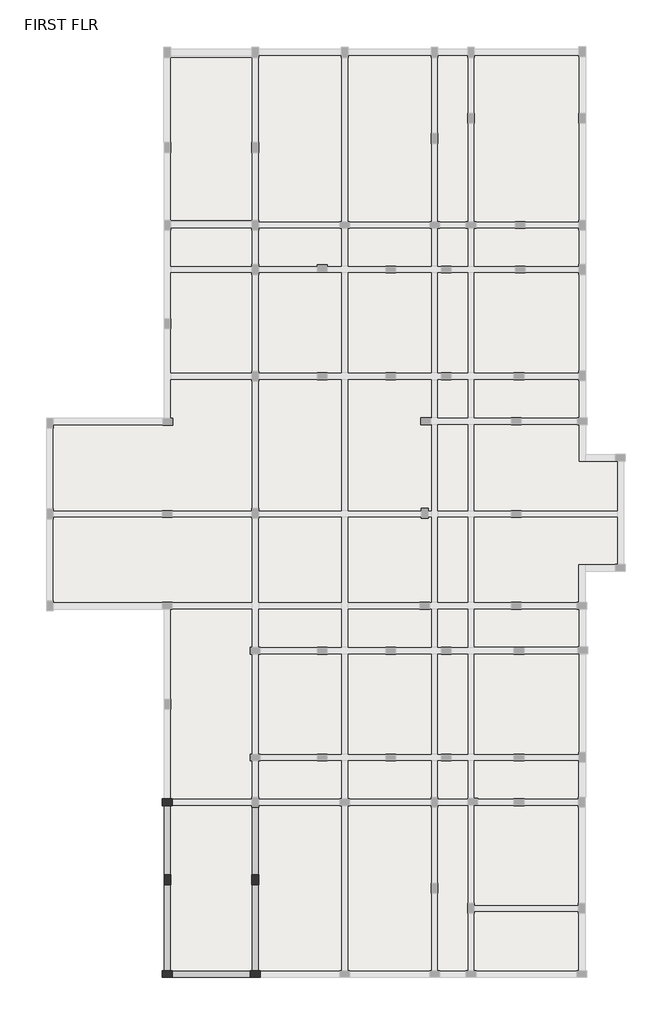
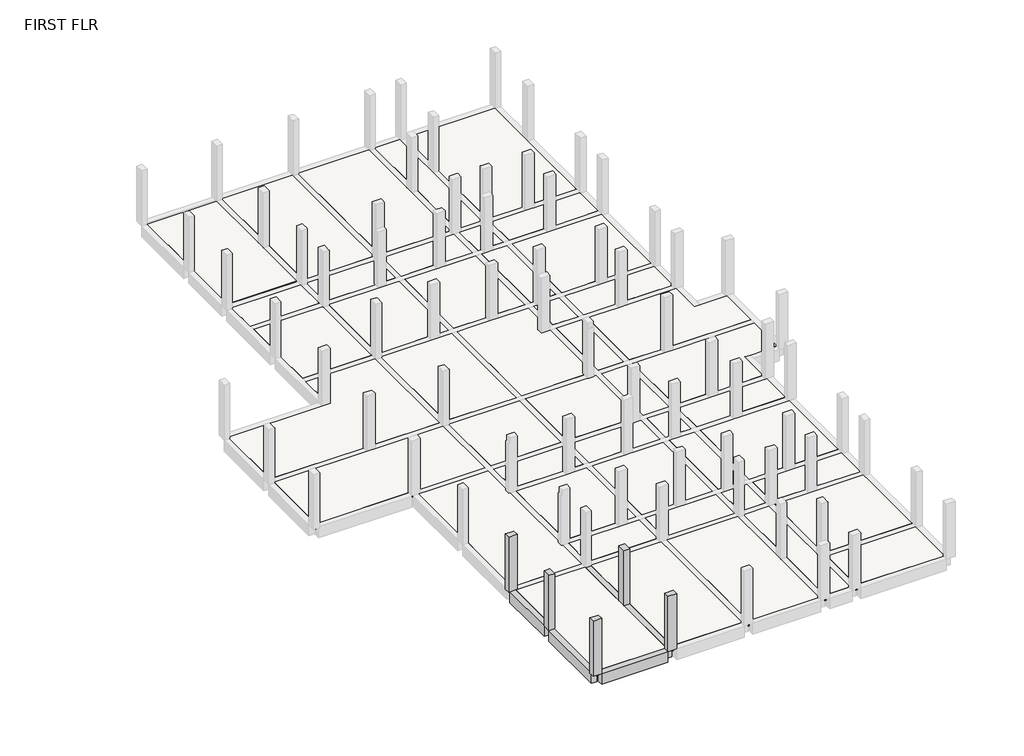
# One storey, part 1 of 5: 5 beams, 5 columns, 2 slabs.
"""IFC4 building model written with IfcOpenShell, lengths in millimetres."""

from ifc_helpers import new_model, si_unit, frame, origin, place, context, project, spatial, polyline, outline, extrude, faceted_brep, element, save

model = new_model("IFC4")

# Units and contexts
model_context = context("Model", 3, world=origin())
ifc_project = project(units=[si_unit("LENGTHUNIT", "METRE", prefix="MILLI")], contexts=[model_context])

# Site, building, storey
site = spatial("IfcSite", under=ifc_project)
building = spatial("IfcBuilding", under=site)
storey = spatial("IfcBuildingStorey", under=building, Name="FIRST FLR", Elevation=3000.0)

# Beams
placement = place(None, origin())
element("IfcBeam", 1, ObjectType="M_Concrete-Rectangular Beam : 300 x 600mm", at=placement, inside=storey, context=model_context, shape_type="Brep", body=[
    faceted_brep([(-5588.8105653, -14991.2517597, 3000.0), (-5588.8105653, -11907.8970059, 3000.0), (-5888.8105653, -11907.8970059, 3000.0), (-5888.8105653, -14991.2517597, 3000.0), (-5888.8105653, -11907.8970059, 2400.0), (-5888.8105653, -14991.2517597, 2400.0), (-5588.8105653, -11907.8970059, 2400.0), (-5588.8105653, -14991.2517597, 2400.0), (-5588.8105653, -14991.2517597, 2700.0), (-5588.8105653, -11907.8970059, 2700.0)], [[[0, 1, 2, 3]], [[3, 2, 4, 5]], [[5, 4, 6, 7]], [[1, 0, 8, 7, 6, 9]], [[6, 4, 2, 1, 9]], [[0, 3, 5, 7, 8]]]),
])
element("IfcBeam", 2, ObjectType="M_Concrete-Rectangular Beam : 300 x 600mm", at=placement, inside=storey, context=model_context, shape_type="Brep", body=[
    faceted_brep([(-5588.8105653, -15441.2517597, 3000.0), (-5888.8105653, -15441.2517597, 3000.0), (-5888.8105653, -19272.5304373, 3000.0), (-5588.8105653, -19272.5304373, 3000.0), (-5888.8105653, -15441.2517597, 2400.0), (-5888.8105653, -19272.5304373, 2400.0), (-5588.8105653, -15441.2517597, 2400.0), (-5588.8105653, -19272.5304373, 2400.0), (-5588.8105653, -19272.5304373, 2700.0), (-5588.8105653, -15441.2517597, 2700.0)], [[[0, 1, 2, 3]], [[1, 4, 5, 2]], [[4, 6, 7, 5]], [[0, 3, 8, 7, 6, 9]], [[6, 4, 1, 0, 9]], [[3, 2, 5, 7, 8]]]),
])
element("IfcBeam", 3, ObjectType="M_Concrete-Rectangular Beam : 300 x 600mm", at=placement, inside=storey, context=model_context, shape_type="SweptSolid", body=[
    extrude(outline(polyline([(-2046.7865686, -19272.5304373), (-2046.7865686, -19572.5304373), (-5516.7865686, -19572.5304373), (-5516.7865686, -19272.5304373), (-2046.7865686, -19272.5304373)])), frame((0.0, 0.0, 2400.0), z_axis=(0.0, 0.0, 1.0), x_axis=(1.0, 0.0, 0.0)), (0.0, 0.0, 1.0), 600.0),
])
element("IfcBeam", 4, ObjectType="M_Concrete-Rectangular Beam : 300 x 600mm", at=placement, inside=storey, context=model_context, shape_type="Brep", body=[
    faceted_brep([(-1971.7865686, -15441.2517597, 3000.0), (-1971.7865686, -19272.5304373, 3000.0), (-1671.7865686, -19272.5304373, 3000.0), (-1671.7865686, -15441.2517597, 3000.0), (-1671.7865686, -19272.5304373, 2700.0), (-1671.7865686, -19272.5304373, 2400.0), (-1671.7865686, -15441.2517597, 2400.0), (-1671.7865686, -15441.2517597, 2700.0), (-1971.7865686, -19272.5304373, 2400.0), (-1971.7865686, -15441.2517597, 2400.0), (-1971.7865686, -15441.2517597, 2700.0), (-1971.7865686, -19272.5304373, 2700.0)], [[[0, 1, 2, 3]], [[3, 2, 4, 5, 6, 7]], [[6, 5, 8, 9]], [[1, 0, 10, 9, 8, 11]], [[0, 3, 7, 6, 9, 10]], [[8, 5, 4, 2, 1, 11]]]),
])
element("IfcBeam", 5, ObjectType="M_Concrete-Rectangular Beam : 300 x 600mm", at=placement, inside=storey, context=model_context, shape_type="Brep", body=[
    faceted_brep([(-1971.7865686, -11982.8970059, 3000.0), (-1971.7865686, -14991.2517597, 3000.0), (-1671.7865686, -14991.2517597, 3000.0), (-1671.7865686, -11982.8970059, 3000.0), (-1671.7865686, -14991.2517597, 2700.0), (-1671.7865686, -14991.2517597, 2400.0), (-1671.7865686, -11982.8970059, 2400.0), (-1671.7865686, -11982.8970059, 2700.0), (-1971.7865686, -14991.2517597, 2400.0), (-1971.7865686, -11982.8970059, 2400.0), (-1971.7865686, -11982.8970059, 2700.0), (-1971.7865686, -14991.2517597, 2700.0)], [[[0, 1, 2, 3]], [[3, 2, 4, 5, 6, 7]], [[6, 5, 8, 9]], [[1, 0, 10, 9, 8, 11]], [[0, 3, 7, 6, 9, 10]], [[8, 5, 4, 2, 1, 11]]]),
])

# Columns
element("IfcColumn", 6, ObjectType="M_Concrete-Rectangular-Column : 300 x 450mm", at=placement, inside=storey, context=model_context, shape_type="Brep", body=[
    faceted_brep([(-5513.8105653, -11907.8970059, 3000.0), (-5963.8105653, -11907.8970059, 3000.0), (-5963.8105653, -11607.8970059, 3000.0), (-5513.8105653, -11607.8970059, 3000.0), (-5513.8105653, -11907.8970059, 5748.0), (-5513.8105653, -11907.8970059, 6048.0), (-5588.8105653, -11907.8970059, 6048.0), (-5963.8105653, -11907.8970059, 6048.0), (-5963.8105653, -11607.8970059, 6048.0), (-5588.8105653, -11607.8970059, 6048.0), (-5513.8105653, -11607.8970059, 6048.0), (-5513.8105653, -11607.8970059, 5748.0)], [[[0, 1, 2, 3]], [[1, 0, 4, 5, 6, 7]], [[2, 1, 7, 8]], [[3, 2, 8, 9, 10, 11]], [[0, 3, 11, 10, 5, 4]], [[8, 7, 6, 5, 10, 9]]]),
])
element("IfcColumn", 7, ObjectType="M_Concrete-Rectangular-Column : 300 x 450mm", at=placement, inside=storey, context=model_context, shape_type="Brep", body=[
    faceted_brep([(-5588.8105653, -14991.2517597, 3000.0), (-5588.8105653, -15441.2517597, 3000.0), (-5888.8105653, -15441.2517597, 3000.0), (-5888.8105653, -14991.2517597, 3000.0), (-5588.8105653, -14991.2517597, 5748.0), (-5588.8105653, -14991.2517597, 6048.0), (-5588.8105653, -15441.2517597, 6048.0), (-5588.8105653, -15441.2517597, 5748.0), (-5888.8105653, -15441.2517597, 6048.0), (-5888.8105653, -14991.2517597, 6048.0)], [[[0, 1, 2, 3]], [[1, 0, 4, 5, 6, 7]], [[2, 1, 7, 6, 8]], [[3, 2, 8, 9]], [[0, 3, 9, 5, 4]], [[6, 5, 9, 8]]]),
])
element("IfcColumn", 8, ObjectType="M_Concrete-Rectangular-Column : 300 x 450mm", at=placement, inside=storey, context=model_context, shape_type="Brep", body=[
    faceted_brep([(-1671.7865686, -14991.2517597, 3000.0), (-1671.7865686, -15441.2517597, 3000.0), (-1971.7865686, -15441.2517597, 3000.0), (-1971.7865686, -14991.2517597, 3000.0), (-1671.7865686, -14991.2517597, 5748.0), (-1671.7865686, -14991.2517597, 6048.0), (-1671.7865686, -15441.2517597, 6048.0), (-1671.7865686, -15441.2517597, 5748.0), (-1971.7865686, -15441.2517597, 6048.0), (-1971.7865686, -15441.2517597, 5748.0), (-1971.7865686, -14991.2517597, 6048.0), (-1971.7865686, -14991.2517597, 5748.0)], [[[0, 1, 2, 3]], [[1, 0, 4, 5, 6, 7]], [[2, 1, 7, 6, 8, 9]], [[3, 2, 9, 8, 10, 11]], [[0, 3, 11, 10, 5, 4]], [[6, 5, 10, 8]]]),
])
element("IfcColumn", 9, ObjectType="M_Concrete-Rectangular-Column : 300 x 450mm", at=placement, inside=storey, context=model_context, shape_type="Brep", body=[
    faceted_brep([(-2046.7865686, -19272.5304373, 3000.0), (-1596.7865686, -19272.5304373, 3000.0), (-1596.7865686, -19572.5304373, 3000.0), (-2046.7865686, -19572.5304373, 3000.0), (-2046.7865686, -19272.5304373, 6048.0), (-1971.7865686, -19272.5304373, 6048.0), (-1671.7865686, -19272.5304373, 6048.0), (-1596.7865686, -19272.5304373, 6048.0), (-1596.7865686, -19572.5304373, 6048.0), (-2046.7865686, -19572.5304373, 6048.0)], [[[0, 1, 2, 3]], [[4, 5, 6, 7, 1, 0]], [[7, 8, 2, 1]], [[8, 9, 3, 2]], [[9, 4, 0, 3]], [[4, 9, 8, 7, 6, 5]]]),
])
element("IfcColumn", 10, ObjectType="M_Concrete-Rectangular-Column : 300 x 450mm", at=placement, inside=storey, context=model_context, shape_type="Brep", body=[
    faceted_brep([(-5516.7865686, -19572.5304373, 3000.0), (-5966.7865686, -19572.5304373, 3000.0), (-5966.7865686, -19272.5304373, 3000.0), (-5516.7865686, -19272.5304373, 3000.0), (-5516.7865686, -19572.5304373, 6048.0), (-5966.7865686, -19572.5304373, 6048.0), (-5966.7865686, -19272.5304373, 6048.0), (-5588.8105653, -19272.5304373, 6048.0), (-5516.7865686, -19272.5304373, 6048.0)], [[[0, 1, 2, 3]], [[4, 5, 1, 0]], [[5, 6, 2, 1]], [[6, 7, 8, 3, 2]], [[8, 4, 0, 3]], [[4, 8, 7, 6, 5]]]),
])

# Slabs
element("IfcSlab", 11, ObjectType="Generic 300mm", at=placement, inside=storey, context=model_context, shape_type="Brep", body=[
    faceted_brep([(-1971.7865686, 21462.8349362, 2700.0), (-1971.7865686, 14212.5179708, 2700.0), (-5588.8105653, 14212.5179708, 2700.0), (-5591.7865686, 14212.5179708, 2700.0), (-5591.7865686, 17224.7148651, 2700.0), (-5591.7865686, 17674.7148651, 2700.0), (-5591.7865686, 21462.8349362, 2700.0), (-1971.7865686, 21462.8349362, 3000.0), (-5591.7865686, 21462.8349362, 3000.0), (-5591.7865686, 17674.7148651, 3000.0), (-5591.7865686, 17224.7148651, 3000.0), (-5591.7865686, 14212.5179708, 3000.0), (-5588.8105653, 14212.5179708, 3000.0), (-1971.7865686, 14212.5179708, 3000.0), (-1971.7865686, 17224.7148651, 3000.0), (-1971.7865686, 17674.7148651, 3000.0)], [[[0, 1, 2, 3, 4, 5, 6]], [[7, 8, 9, 10, 11, 12, 13, 14, 15]], [[1, 0, 7, 15, 14, 13]], [[3, 2, 1, 13, 12, 11]], [[6, 5, 4, 3, 11, 10, 9, 8]], [[0, 6, 8, 7]]]),
    faceted_brep([(2024.7296816, 21537.8349362, 2700.0), (2024.7296816, 14137.5179708, 2700.0), (-1671.7865686, 14137.5179708, 2700.0), (-1671.7865686, 21537.8349362, 2700.0), (2024.7296816, 21537.8349362, 3000.0), (-1671.7865686, 21537.8349362, 3000.0), (-1671.7865686, 21462.8349362, 3000.0), (-1671.7865686, 17674.7148651, 3000.0), (-1671.7865686, 17224.7148651, 3000.0), (-1671.7865686, 14212.5179708, 3000.0), (-1671.7865686, 14137.5179708, 3000.0), (1949.7296816, 14137.5179708, 3000.0), (2024.7296816, 14137.5179708, 3000.0), (2024.7296816, 21462.8349362, 3000.0)], [[[0, 1, 2, 3]], [[4, 5, 6, 7, 8, 9, 10, 11, 12, 13]], [[1, 0, 4, 13, 12]], [[2, 1, 12, 11, 10]], [[3, 2, 10, 9, 8, 7, 6, 5]], [[0, 3, 5, 4]]]),
    faceted_brep([(6032.5248054, 21537.8349362, 2700.0), (6032.5248054, 14137.5179708, 2700.0), (2324.7296816, 14137.5179708, 2700.0), (2324.7296816, 21537.8349362, 2700.0), (6032.5248054, 21537.8349362, 3000.0), (2324.7296816, 21537.8349362, 3000.0), (2324.7296816, 21462.8349362, 3000.0), (2324.7296816, 14137.5179708, 3000.0), (2399.7296816, 14137.5179708, 3000.0), (5957.5248054, 14137.5179708, 3000.0), (6032.5248054, 14137.5179708, 3000.0), (6032.5248054, 17624.7148651, 3000.0), (6032.5248054, 18074.7148651, 3000.0), (6032.5248054, 21462.8349362, 3000.0)], [[[0, 1, 2, 3]], [[4, 5, 6, 7, 8, 9, 10, 11, 12, 13]], [[1, 0, 4, 13, 12, 11, 10]], [[2, 1, 10, 9, 8, 7]], [[3, 2, 7, 6, 5]], [[0, 3, 5, 4]]]),
    faceted_brep([(7656.8679014, 21537.8349362, 2700.0), (7656.8679014, 14137.5179708, 2700.0), (6332.5248054, 14137.5179708, 2700.0), (6332.5248054, 21537.8349362, 2700.0), (7656.8679014, 21537.8349362, 3000.0), (6332.5248054, 21537.8349362, 3000.0), (6332.5248054, 21462.8349362, 3000.0), (6332.5248054, 18074.7148651, 3000.0), (6332.5248054, 17624.7148651, 3000.0), (6332.5248054, 14137.5179708, 3000.0), (6407.5248054, 14137.5179708, 3000.0), (7581.8679014, 14137.5179708, 3000.0), (7656.8679014, 14137.5179708, 3000.0), (7656.8679014, 18524.7148651, 3000.0), (7656.8679014, 18974.7148651, 3000.0), (7656.8679014, 21462.8349362, 3000.0)], [[[0, 1, 2, 3]], [[4, 5, 6, 7, 8, 9, 10, 11, 12, 13, 14, 15]], [[1, 0, 4, 15, 14, 13, 12]], [[2, 1, 12, 11, 10, 9]], [[3, 2, 9, 8, 7, 6, 5]], [[0, 3, 5, 4]]]),
    faceted_brep([(12619.1163908, 21537.8349362, 2700.0), (12619.1163908, 14137.5179708, 2700.0), (7956.8679014, 14137.5179708, 2700.0), (7956.8679014, 21537.8349362, 2700.0), (12619.1163908, 21537.8349362, 3000.0), (7956.8679014, 21537.8349362, 3000.0), (7956.8679014, 21462.8349362, 3000.0), (7956.8679014, 18974.7148651, 3000.0), (7956.8679014, 18524.7148651, 3000.0), (7956.8679014, 14137.5179708, 3000.0), (8031.8679014, 14137.5179708, 3000.0), (9781.8679014, 14137.5179708, 3000.0), (10231.8679014, 14137.5179708, 3000.0), (12619.1163908, 14137.5179708, 3000.0), (12619.1163908, 14212.5179708, 3000.0), (12619.1163908, 18524.7148651, 3000.0), (12619.1163908, 18974.7148651, 3000.0), (12619.1163908, 21502.8349362, 3000.0)], [[[0, 1, 2, 3]], [[4, 5, 6, 7, 8, 9, 10, 11, 12, 13, 14, 15, 16, 17]], [[1, 0, 4, 17, 16, 15, 14, 13]], [[2, 1, 13, 12, 11, 10, 9]], [[3, 2, 9, 8, 7, 6, 5]], [[0, 3, 5, 4]]]),
    faceted_brep([(-1971.7865686, 13837.5179708, 2700.0), (-1971.7865686, 12157.4075451, 2700.0), (-5588.8105653, 12157.4075451, 2700.0), (-5588.8105653, 13837.5179708, 2700.0), (-1971.7865686, 13837.5179708, 3000.0), (-5588.8105653, 13837.5179708, 3000.0), (-5588.8105653, 13762.5179708, 3000.0), (-5588.8105653, 12157.4075451, 3000.0), (-1971.7865686, 12157.4075451, 3000.0), (-1971.7865686, 12232.4075451, 3000.0), (-1971.7865686, 13762.5179708, 3000.0)], [[[0, 1, 2, 3]], [[4, 5, 6, 7, 8, 9, 10]], [[1, 0, 4, 10, 9, 8]], [[2, 1, 8, 7]], [[3, 2, 7, 6, 5]], [[0, 3, 5, 4]]]),
    faceted_brep([(2024.7296816, 13837.5179708, 2700.0), (2024.7296816, 12157.4075451, 2700.0), (1399.7296816, 12157.4075451, 2700.0), (949.7296816, 12157.4075451, 2700.0), (-1671.7865686, 12157.4075451, 2700.0), (-1671.7865686, 13837.5179708, 2700.0), (2024.7296816, 13837.5179708, 3000.0), (1949.7296816, 13837.5179708, 3000.0), (-1671.7865686, 13837.5179708, 3000.0), (-1671.7865686, 13762.5179708, 3000.0), (-1671.7865686, 12232.4075451, 3000.0), (-1671.7865686, 12157.4075451, 3000.0), (949.7296816, 12157.4075451, 3000.0), (1399.7296816, 12157.4075451, 3000.0), (2024.7296816, 12157.4075451, 3000.0)], [[[0, 1, 2, 3, 4, 5]], [[6, 7, 8, 9, 10, 11, 12, 13, 14]], [[1, 0, 6, 14]], [[4, 3, 2, 1, 14, 13, 12, 11]], [[5, 4, 11, 10, 9, 8]], [[0, 5, 8, 7, 6]]]),
    faceted_brep([(6032.5248054, 13837.5179708, 2700.0), (6032.5248054, 12157.4075451, 2700.0), (2324.7296816, 12157.4075451, 2700.0), (2324.7296816, 13837.5179708, 2700.0), (6032.5248054, 13837.5179708, 3000.0), (5957.5248054, 13837.5179708, 3000.0), (2399.7296816, 13837.5179708, 3000.0), (2324.7296816, 13837.5179708, 3000.0), (2324.7296816, 12157.4075451, 3000.0), (3997.5248054, 12157.4075451, 3000.0), (4447.5248054, 12157.4075451, 3000.0), (6032.5248054, 12157.4075451, 3000.0)], [[[0, 1, 2, 3]], [[4, 5, 6, 7, 8, 9, 10, 11]], [[1, 0, 4, 11]], [[2, 1, 11, 10, 9, 8]], [[3, 2, 8, 7]], [[0, 3, 7, 6, 5, 4]]]),
    faceted_brep([(7656.8679014, 13837.5179708, 2700.0), (7656.8679014, 12157.4075451, 2700.0), (6332.5248054, 12157.4075451, 2700.0), (6332.5248054, 13837.5179708, 2700.0), (7656.8679014, 13837.5179708, 3000.0), (7581.8679014, 13837.5179708, 3000.0), (6407.5248054, 13837.5179708, 3000.0), (6332.5248054, 13837.5179708, 3000.0), (6332.5248054, 12157.4075451, 3000.0), (6481.8679014, 12157.4075451, 3000.0), (6931.8679014, 12157.4075451, 3000.0), (7656.8679014, 12157.4075451, 3000.0)], [[[0, 1, 2, 3]], [[4, 5, 6, 7, 8, 9, 10, 11]], [[1, 0, 4, 11]], [[2, 1, 11, 10, 9, 8]], [[3, 2, 8, 7]], [[0, 3, 7, 6, 5, 4]]]),
    faceted_brep([(12619.1163908, 13837.5179708, 2700.0), (12619.1163908, 12157.4075451, 2700.0), (7956.8679014, 12157.4075451, 2700.0), (7956.8679014, 13837.5179708, 2700.0), (12619.1163908, 13837.5179708, 3000.0), (10231.8679014, 13837.5179708, 3000.0), (9781.8679014, 13837.5179708, 3000.0), (8031.8679014, 13837.5179708, 3000.0), (7956.8679014, 13837.5179708, 3000.0), (7956.8679014, 12157.4075451, 3000.0), (9781.8679014, 12157.4075451, 3000.0), (10231.8679014, 12157.4075451, 3000.0), (12619.1163908, 12157.4075451, 3000.0), (12619.1163908, 12232.4075451, 3000.0), (12619.1163908, 13762.5179708, 3000.0)], [[[0, 1, 2, 3]], [[4, 5, 6, 7, 8, 9, 10, 11, 12, 13, 14]], [[1, 0, 4, 14, 13, 12]], [[2, 1, 12, 11, 10, 9]], [[3, 2, 9, 8]], [[0, 3, 8, 7, 6, 5, 4]]]),
    faceted_brep([(-1971.7865686, 11857.4075451, 2700.0), (-1971.7865686, 7399.7076276, 2700.0), (-5588.8105653, 7399.7076276, 2700.0), (-5588.8105653, 11857.4075451, 2700.0), (-1971.7865686, 11857.4075451, 3000.0), (-5588.8105653, 11857.4075451, 3000.0), (-5588.8105653, 9817.5252033, 3000.0), (-5588.8105653, 9367.5252033, 3000.0), (-5588.8105653, 7399.7076276, 3000.0), (-1971.7865686, 7399.7076276, 3000.0), (-1971.7865686, 7474.7076276, 3000.0), (-1971.7865686, 11782.4075451, 3000.0)], [[[0, 1, 2, 3]], [[4, 5, 6, 7, 8, 9, 10, 11]], [[1, 0, 4, 11, 10, 9]], [[2, 1, 9, 8]], [[3, 2, 8, 7, 6, 5]], [[0, 3, 5, 4]]]),
    faceted_brep([(2024.7296816, 11857.4075451, 2700.0), (2024.7296816, 7399.7076276, 2700.0), (-1671.7865686, 7399.7076276, 2700.0), (-1671.7865686, 11857.4075451, 2700.0), (2024.7296816, 11857.4075451, 3000.0), (-1671.7865686, 11857.4075451, 3000.0), (-1671.7865686, 11782.4075451, 3000.0), (-1671.7865686, 7474.7076276, 3000.0), (-1671.7865686, 7399.7076276, 3000.0), (949.7296816, 7399.7076276, 3000.0), (1399.7296816, 7399.7076276, 3000.0), (2024.7296816, 7399.7076276, 3000.0)], [[[0, 1, 2, 3]], [[4, 5, 6, 7, 8, 9, 10, 11]], [[1, 0, 4, 11]], [[2, 1, 11, 10, 9, 8]], [[3, 2, 8, 7, 6, 5]], [[0, 3, 5, 4]]]),
    faceted_brep([(6032.5248054, 11857.4075451, 2700.0), (6032.5248054, 7399.7076276, 2700.0), (2324.7296816, 7399.7076276, 2700.0), (2324.7296816, 11857.4075451, 2700.0), (6032.5248054, 11857.4075451, 3000.0), (4447.5248054, 11857.4075451, 3000.0), (3997.5248054, 11857.4075451, 3000.0), (2324.7296816, 11857.4075451, 3000.0), (2324.7296816, 7399.7076276, 3000.0), (3997.5248054, 7399.7076276, 3000.0), (4447.5248054, 7399.7076276, 3000.0), (6032.5248054, 7399.7076276, 3000.0)], [[[0, 1, 2, 3]], [[4, 5, 6, 7, 8, 9, 10, 11]], [[1, 0, 4, 11]], [[2, 1, 11, 10, 9, 8]], [[3, 2, 8, 7]], [[0, 3, 7, 6, 5, 4]]]),
    faceted_brep([(7656.8679014, 11857.4075451, 2700.0), (7656.8679014, 7399.7076276, 2700.0), (6332.5248054, 7399.7076276, 2700.0), (6332.5248054, 11857.4075451, 2700.0), (7656.8679014, 11857.4075451, 3000.0), (6931.8679014, 11857.4075451, 3000.0), (6481.8679014, 11857.4075451, 3000.0), (6332.5248054, 11857.4075451, 3000.0), (6332.5248054, 7399.7076276, 3000.0), (6481.8679014, 7399.7076276, 3000.0), (6931.8679014, 7399.7076276, 3000.0), (7656.8679014, 7399.7076276, 3000.0)], [[[0, 1, 2, 3]], [[4, 5, 6, 7, 8, 9, 10, 11]], [[1, 0, 4, 11]], [[2, 1, 11, 10, 9, 8]], [[3, 2, 8, 7]], [[0, 3, 7, 6, 5, 4]]]),
    faceted_brep([(12616.8679014, 11857.4075451, 2700.0), (12616.8679014, 7399.7076276, 2700.0), (7956.8679014, 7399.7076276, 2700.0), (7956.8679014, 11857.4075451, 2700.0), (12616.8679014, 11857.4075451, 3000.0), (10231.8679014, 11857.4075451, 3000.0), (9781.8679014, 11857.4075451, 3000.0), (7956.8679014, 11857.4075451, 3000.0), (7956.8679014, 7399.7076276, 3000.0), (9721.8679014, 7399.7076276, 3000.0), (10171.8679014, 7399.7076276, 3000.0), (12616.8679014, 7399.7076276, 3000.0)], [[[0, 1, 2, 3]], [[4, 5, 6, 7, 8, 9, 10, 11]], [[1, 0, 4, 11]], [[2, 1, 11, 10, 9, 8]], [[3, 2, 8, 7]], [[0, 3, 7, 6, 5, 4]]]),
    faceted_brep([(7656.8679014, 7099.7076276, 2700.0), (7656.8679014, 5387.6057249, 2700.0), (6332.5248054, 5387.6057249, 2700.0), (6332.5248054, 7099.7076276, 2700.0), (7656.8679014, 7099.7076276, 3000.0), (6931.8679014, 7099.7076276, 3000.0), (6481.8679014, 7099.7076276, 3000.0), (6332.5248054, 7099.7076276, 3000.0), (6332.5248054, 5387.6057249, 3000.0), (7656.8679014, 5387.6057249, 3000.0)], [[[0, 1, 2, 3]], [[4, 5, 6, 7, 8, 9]], [[1, 0, 4, 9]], [[2, 1, 9, 8]], [[3, 2, 8, 7]], [[0, 3, 7, 6, 5, 4]]]),
    faceted_brep([(12616.8679014, 7099.7076276, 2700.0), (12616.8679014, 5387.6057249, 2700.0), (7956.8679014, 5387.6057249, 2700.0), (7956.8679014, 7099.7076276, 2700.0), (12616.8679014, 7099.7076276, 3000.0), (10171.8679014, 7099.7076276, 3000.0), (9721.8679014, 7099.7076276, 3000.0), (7956.8679014, 7099.7076276, 3000.0), (7956.8679014, 5387.6057249, 3000.0), (9601.8679014, 5387.6057249, 3000.0), (10051.8679014, 5387.6057249, 3000.0), (12541.8679014, 5387.6057249, 3000.0), (12616.8679014, 5387.6057249, 3000.0)], [[[0, 1, 2, 3]], [[4, 5, 6, 7, 8, 9, 10, 11, 12]], [[1, 0, 4, 12]], [[2, 1, 12, 11, 10, 9, 8]], [[3, 2, 8, 7]], [[0, 3, 7, 6, 5, 4]]]),
    faceted_brep([(7656.8679014, 5087.6057249, 2700.0), (7656.8679014, 1251.1713929, 2700.0), (6332.5248054, 1251.1713929, 2700.0), (6332.5248054, 5087.6057249, 2700.0), (7656.8679014, 5087.6057249, 3000.0), (6332.5248054, 5087.6057249, 3000.0), (6332.5248054, 1251.1713929, 3000.0), (7656.8679014, 1251.1713929, 3000.0)], [[[0, 1, 2, 3]], [[4, 5, 6, 7]], [[1, 0, 4, 7]], [[2, 1, 7, 6]], [[3, 2, 6, 5]], [[0, 3, 5, 4]]]),
    faceted_brep([(14319.1163908, 1251.1713929, 2700.0), (7956.8679014, 1251.1713929, 2700.0), (7956.8679014, 5087.6057249, 2700.0), (12616.8679014, 5087.6057249, 2700.0), (12616.8679014, 3435.7536525, 2700.0), (14319.1163908, 3435.7536525, 2700.0), (14319.1163908, 1251.1713929, 3000.0), (14319.1163908, 3435.7536525, 3000.0), (12916.8679014, 3435.7536525, 3000.0), (12616.8679014, 3435.7536525, 3000.0), (12616.8679014, 5087.6057249, 3000.0), (12541.8679014, 5087.6057249, 3000.0), (10051.8679014, 5087.6057249, 3000.0), (9601.8679014, 5087.6057249, 3000.0), (7956.8679014, 5087.6057249, 3000.0), (7956.8679014, 1251.1713929, 3000.0), (9601.8679014, 1251.1713929, 3000.0), (10051.8679014, 1251.1713929, 3000.0)], [[[0, 1, 2, 3, 4, 5]], [[6, 7, 8, 9, 10, 11, 12, 13, 14, 15, 16, 17]], [[1, 0, 6, 17, 16, 15]], [[2, 1, 15, 14]], [[3, 2, 14, 13, 12, 11, 10]], [[4, 3, 10, 9]], [[5, 4, 9, 8, 7]], [[0, 5, 7, 6]]]),
    faceted_brep([(7956.8679014, -2839.4535766, 2700.0), (7956.8679014, 951.1713929, 2700.0), (14319.1163908, 951.1713929, 2700.0), (14319.1163908, -1148.8286071, 2700.0), (12599.1163908, -1148.8286071, 2700.0), (12599.1163908, -2839.4535766, 2700.0), (7956.8679014, -2839.4535766, 3000.0), (9601.8679014, -2839.4535766, 3000.0), (10051.8679014, -2839.4535766, 3000.0), (12524.1163908, -2839.4535766, 3000.0), (12599.1163908, -2839.4535766, 3000.0), (12599.1163908, -1148.8286071, 3000.0), (12899.1163908, -1148.8286071, 3000.0), (14244.1163908, -1148.8286071, 3000.0), (14319.1163908, -1148.8286071, 3000.0), (14319.1163908, 951.1713929, 3000.0), (10051.8679014, 951.1713929, 3000.0), (9601.8679014, 951.1713929, 3000.0), (7956.8679014, 951.1713929, 3000.0)], [[[0, 1, 2, 3, 4, 5]], [[6, 7, 8, 9, 10, 11, 12, 13, 14, 15, 16, 17, 18]], [[1, 0, 6, 18]], [[2, 1, 18, 17, 16, 15]], [[3, 2, 15, 14]], [[4, 3, 14, 13, 12, 11]], [[5, 4, 11, 10]], [[0, 5, 10, 9, 8, 7, 6]]]),
    faceted_brep([(7656.8679014, 951.1713929, 2700.0), (7656.8679014, -2839.4535766, 2700.0), (6332.5248054, -2839.4535766, 2700.0), (6332.5248054, 951.1713929, 2700.0), (7656.8679014, 951.1713929, 3000.0), (6332.5248054, 951.1713929, 3000.0), (6332.5248054, -2839.4535766, 3000.0), (7656.8679014, -2839.4535766, 3000.0)], [[[0, 1, 2, 3]], [[4, 5, 6, 7]], [[1, 0, 4, 7]], [[2, 1, 7, 6]], [[3, 2, 6, 5]], [[0, 3, 5, 4]]]),
    faceted_brep([(6032.5248054, 951.1713929, 2700.0), (6032.5248054, -2839.4535766, 2700.0), (2324.7296816, -2839.4535766, 2700.0), (2324.7296816, 951.1713929, 2700.0), (5592.5248054, 951.1713929, 2700.0), (5892.5248054, 951.1713929, 2700.0), (6032.5248054, 951.1713929, 3000.0), (5892.5248054, 951.1713929, 3000.0), (5592.5248054, 951.1713929, 3000.0), (2324.7296816, 951.1713929, 3000.0), (2324.7296816, -2839.4535766, 3000.0), (5517.5248054, -2839.4535766, 3000.0), (5967.5248054, -2839.4535766, 3000.0), (6032.5248054, -2839.4535766, 3000.0)], [[[0, 1, 2, 3, 4, 5]], [[6, 7, 8, 9, 10, 11, 12, 13]], [[1, 0, 6, 13]], [[2, 1, 13, 12, 11, 10]], [[3, 2, 10, 9]], [[0, 5, 4, 3, 9, 8, 7, 6]]]),
    faceted_brep([(2024.7296816, 951.1713929, 2700.0), (2024.7296816, -2839.4535766, 2700.0), (-1671.7865686, -2839.4535766, 2700.0), (-1671.7865686, 951.1713929, 2700.0), (2024.7296816, 951.1713929, 3000.0), (-1671.7865686, 951.1713929, 3000.0), (-1671.7865686, 916.1713929, 3000.0), (-1671.7865686, -2839.4535766, 3000.0), (2024.7296816, -2839.4535766, 3000.0)], [[[0, 1, 2, 3]], [[4, 5, 6, 7, 8]], [[1, 0, 4, 8]], [[2, 1, 8, 7]], [[3, 2, 7, 6, 5]], [[0, 3, 5, 4]]]),
    faceted_brep([(2024.7296816, 7099.7076276, 2700.0), (2024.7296816, 1251.1713929, 2700.0), (-1671.7865686, 1251.1713929, 2700.0), (-1671.7865686, 7099.7076276, 2700.0), (2024.7296816, 7099.7076276, 3000.0), (1399.7296816, 7099.7076276, 3000.0), (949.7296816, 7099.7076276, 3000.0), (-1671.7865686, 7099.7076276, 3000.0), (-1671.7865686, 7024.7076276, 3000.0), (-1671.7865686, 1366.1713929, 3000.0), (-1671.7865686, 1251.1713929, 3000.0), (2024.7296816, 1251.1713929, 3000.0)], [[[0, 1, 2, 3]], [[4, 5, 6, 7, 8, 9, 10, 11]], [[1, 0, 4, 11]], [[2, 1, 11, 10]], [[3, 2, 10, 9, 8, 7]], [[0, 3, 7, 6, 5, 4]]]),
    faceted_brep([(-10828.8105653, 1251.1713929, 2700.0), (-10828.8105653, 5067.6057249, 2700.0), (-5493.8105653, 5067.6057249, 2700.0), (-5493.8105653, 5367.5252033, 2700.0), (-5588.8105653, 5367.5252033, 2700.0), (-5588.8105653, 7099.7076276, 2700.0), (-1971.7865686, 7099.7076276, 2700.0), (-1971.7865686, 1251.1713929, 2700.0), (-10828.8105653, 1251.1713929, 3000.0), (-5963.8105653, 1251.1713929, 3000.0), (-5513.8105653, 1251.1713929, 3000.0), (-1971.7865686, 1251.1713929, 3000.0), (-1971.7865686, 1366.1713929, 3000.0), (-1971.7865686, 7024.7076276, 3000.0), (-1971.7865686, 7099.7076276, 3000.0), (-5588.8105653, 7099.7076276, 3000.0), (-5588.8105653, 5367.5252033, 3000.0), (-5493.8105653, 5367.5252033, 3000.0), (-5493.8105653, 5067.6057249, 3000.0), (-5943.8105653, 5067.6057249, 3000.0), (-10828.8105653, 5067.6057249, 3000.0), (-10828.8105653, 4932.6057249, 3000.0), (-10828.8105653, 1326.1713929, 3000.0)], [[[0, 1, 2, 3, 4, 5, 6, 7]], [[8, 9, 10, 11, 12, 13, 14, 15, 16, 17, 18, 19, 20, 21, 22]], [[1, 0, 8, 22, 21, 20]], [[2, 1, 20, 19, 18]], [[3, 2, 18, 17]], [[4, 3, 17, 16]], [[5, 4, 16, 15]], [[6, 5, 15, 14]], [[7, 6, 14, 13, 12, 11]], [[0, 7, 11, 10, 9, 8]]]),
    faceted_brep([(-1971.7865686, -2839.4535766, 2700.0), (-10828.8105653, -2839.4535766, 2700.0), (-10828.8105653, 951.1713929, 2700.0), (-1971.7865686, 951.1713929, 2700.0), (-1971.7865686, -2839.4535766, 3000.0), (-1971.7865686, 916.1713929, 3000.0), (-1971.7865686, 951.1713929, 3000.0), (-5513.8105653, 951.1713929, 3000.0), (-5963.8105653, 951.1713929, 3000.0), (-10828.8105653, 951.1713929, 3000.0), (-10828.8105653, 876.1713929, 3000.0), (-10828.8105653, -2764.4535766, 3000.0), (-10828.8105653, -2839.4535766, 3000.0), (-5963.8105653, -2839.4535766, 3000.0), (-5513.8105653, -2839.4535766, 3000.0)], [[[0, 1, 2, 3]], [[4, 5, 6, 7, 8, 9, 10, 11, 12, 13, 14]], [[1, 0, 4, 14, 13, 12]], [[2, 1, 12, 11, 10, 9]], [[3, 2, 9, 8, 7, 6]], [[0, 3, 6, 5, 4]]]),
    faceted_brep([(2024.7296816, -3139.4535766, 2700.0), (2024.7296816, -4851.6229916, 2700.0), (-1671.7865686, -4851.6229916, 2700.0), (-1671.7865686, -3139.4535766, 2700.0), (2024.7296816, -3139.4535766, 3000.0), (-1671.7865686, -3139.4535766, 3000.0), (-1671.7865686, -4851.6229916, 3000.0), (-1596.7865686, -4851.6229916, 3000.0), (949.7296816, -4851.6229916, 3000.0), (1399.7296816, -4851.6229916, 3000.0), (2024.7296816, -4851.6229916, 3000.0)], [[[0, 1, 2, 3]], [[4, 5, 6, 7, 8, 9, 10]], [[1, 0, 4, 10]], [[2, 1, 10, 9, 8, 7, 6]], [[3, 2, 6, 5]], [[0, 3, 5, 4]]]),
    faceted_brep([(6032.5248054, -3139.4535766, 2700.0), (6032.5248054, -4851.6229916, 2700.0), (2324.7296816, -4851.6229916, 2700.0), (2324.7296816, -3139.4535766, 2700.0), (6032.5248054, -3139.4535766, 3000.0), (5967.5248054, -3139.4535766, 3000.0), (5517.5248054, -3139.4535766, 3000.0), (2324.7296816, -3139.4535766, 3000.0), (2324.7296816, -4851.6229916, 3000.0), (3997.5248054, -4851.6229916, 3000.0), (4447.5248054, -4851.6229916, 3000.0), (6032.5248054, -4851.6229916, 3000.0)], [[[0, 1, 2, 3]], [[4, 5, 6, 7, 8, 9, 10, 11]], [[1, 0, 4, 11]], [[2, 1, 11, 10, 9, 8]], [[3, 2, 8, 7]], [[0, 3, 7, 6, 5, 4]]]),
    faceted_brep([(2024.7296816, -5151.6229916, 2700.0), (2024.7296816, -9607.1078267, 2700.0), (-1671.7865686, -9607.1078267, 2700.0), (-1671.7865686, -5151.6229916, 2700.0), (2024.7296816, -5151.6229916, 3000.0), (1399.7296816, -5151.6229916, 3000.0), (949.7296816, -5151.6229916, 3000.0), (-1596.7865686, -5151.6229916, 3000.0), (-1671.7865686, -5151.6229916, 3000.0), (-1671.7865686, -9607.1078267, 3000.0), (-1596.7865686, -9607.1078267, 3000.0), (949.7296816, -9607.1078267, 3000.0), (1399.7296816, -9607.1078267, 3000.0), (2024.7296816, -9607.1078267, 3000.0)], [[[0, 1, 2, 3]], [[4, 5, 6, 7, 8, 9, 10, 11, 12, 13]], [[1, 0, 4, 13]], [[2, 1, 13, 12, 11, 10, 9]], [[3, 2, 9, 8]], [[0, 3, 8, 7, 6, 5, 4]]]),
    faceted_brep([(6032.5248054, -5151.6229916, 2700.0), (6032.5248054, -9607.1078267, 2700.0), (2324.7296816, -9607.1078267, 2700.0), (2324.7296816, -5151.6229916, 2700.0), (6032.5248054, -5151.6229916, 3000.0), (4447.5248054, -5151.6229916, 3000.0), (3997.5248054, -5151.6229916, 3000.0), (2324.7296816, -5151.6229916, 3000.0), (2324.7296816, -9607.1078267, 3000.0), (3997.5248054, -9607.1078267, 3000.0), (4447.5248054, -9607.1078267, 3000.0), (6032.5248054, -9607.1078267, 3000.0)], [[[0, 1, 2, 3]], [[4, 5, 6, 7, 8, 9, 10, 11]], [[1, 0, 4, 11]], [[2, 1, 11, 10, 9, 8]], [[3, 2, 8, 7]], [[0, 3, 7, 6, 5, 4]]]),
    faceted_brep([(7656.8679014, -5151.6229916, 2700.0), (7656.8679014, -9607.1078267, 2700.0), (6332.5248054, -9607.1078267, 2700.0), (6332.5248054, -5151.6229916, 2700.0), (7656.8679014, -5151.6229916, 3000.0), (6931.8679014, -5151.6229916, 3000.0), (6481.8679014, -5151.6229916, 3000.0), (6332.5248054, -5151.6229916, 3000.0), (6332.5248054, -9607.1078267, 3000.0), (6481.8679014, -9607.1078267, 3000.0), (6931.8679014, -9607.1078267, 3000.0), (7656.8679014, -9607.1078267, 3000.0)], [[[0, 1, 2, 3]], [[4, 5, 6, 7, 8, 9, 10, 11]], [[1, 0, 4, 11]], [[2, 1, 11, 10, 9, 8]], [[3, 2, 8, 7]], [[0, 3, 7, 6, 5, 4]]]),
    faceted_brep([(12619.1163908, -3139.4535766, 2700.0), (12619.1163908, -4831.6229916, 2700.0), (7956.8679014, -4831.6229916, 2700.0), (7956.8679014, -3139.4535766, 2700.0), (12619.1163908, -3139.4535766, 3000.0), (12524.1163908, -3139.4535766, 3000.0), (10051.8679014, -3139.4535766, 3000.0), (9601.8679014, -3139.4535766, 3000.0), (7956.8679014, -3139.4535766, 3000.0), (7956.8679014, -4831.6229916, 3000.0), (12564.1163908, -4831.6229916, 3000.0), (12619.1163908, -4831.6229916, 3000.0), (12619.1163908, -4818.9229916, 3000.0)], [[[0, 1, 2, 3]], [[4, 5, 6, 7, 8, 9, 10, 11, 12]], [[1, 0, 4, 12, 11]], [[2, 1, 11, 10, 9]], [[3, 2, 9, 8]], [[0, 3, 8, 7, 6, 5, 4]]]),
    faceted_brep([(12619.1163908, -5151.6229916, 2700.0), (12619.1163908, -9607.1078267, 2700.0), (7956.8679014, -9607.1078267, 2700.0), (7956.8679014, -5151.6229916, 2700.0), (12619.1163908, -5151.6229916, 3000.0), (10171.8679014, -5151.6229916, 3000.0), (9721.8679014, -5151.6229916, 3000.0), (7956.8679014, -5151.6229916, 3000.0), (7956.8679014, -9607.1078267, 3000.0), (9721.8679014, -9607.1078267, 3000.0), (10171.8679014, -9607.1078267, 3000.0), (12619.1163908, -9607.1078267, 3000.0), (12619.1163908, -9532.1078267, 3000.0)], [[[0, 1, 2, 3]], [[4, 5, 6, 7, 8, 9, 10, 11, 12]], [[1, 0, 4, 12, 11]], [[2, 1, 11, 10, 9, 8]], [[3, 2, 8, 7]], [[0, 3, 7, 6, 5, 4]]]),
    faceted_brep([(12599.1163908, -9907.1078267, 2700.0), (12599.1163908, -11607.8970059, 2700.0), (8111.8679014, -11607.8970059, 2700.0), (7956.8679014, -11607.8970059, 2700.0), (7956.8679014, -11587.8970059, 2700.0), (7956.8679014, -9907.1078267, 2700.0), (12599.1163908, -9907.1078267, 3000.0), (10171.8679014, -9907.1078267, 3000.0), (9721.8679014, -9907.1078267, 3000.0), (7956.8679014, -9907.1078267, 3000.0), (7956.8679014, -11587.8970059, 3000.0), (7956.8679014, -11607.8970059, 3000.0), (8111.8679014, -11607.8970059, 3000.0), (9721.8679014, -11607.8970059, 3000.0), (10171.8679014, -11607.8970059, 3000.0), (12599.1163908, -11607.8970059, 3000.0), (12599.1163908, -11532.8970059, 3000.0)], [[[0, 1, 2, 3, 4, 5]], [[6, 7, 8, 9, 10, 11, 12, 13, 14, 15, 16]], [[1, 0, 6, 16, 15]], [[3, 2, 1, 15, 14, 13, 12, 11]], [[5, 4, 3, 11, 10, 9]], [[0, 5, 9, 8, 7, 6]]]),
    faceted_brep([(7656.8679014, -9907.1078267, 2700.0), (7656.8679014, -11607.8970059, 2700.0), (6332.5248054, -11607.8970059, 2700.0), (6332.5248054, -9907.1078267, 2700.0), (7656.8679014, -9907.1078267, 3000.0), (6931.8679014, -9907.1078267, 3000.0), (6481.8679014, -9907.1078267, 3000.0), (6332.5248054, -9907.1078267, 3000.0), (6332.5248054, -11532.8970059, 3000.0), (6332.5248054, -11607.8970059, 3000.0), (7656.8679014, -11607.8970059, 3000.0)], [[[0, 1, 2, 3]], [[4, 5, 6, 7, 8, 9, 10]], [[1, 0, 4, 10]], [[2, 1, 10, 9]], [[3, 2, 9, 8, 7]], [[0, 3, 7, 6, 5, 4]]]),
    faceted_brep([(6032.5248054, -9907.1078267, 2700.0), (6032.5248054, -11607.8970059, 2700.0), (2324.7296816, -11607.8970059, 2700.0), (2324.7296816, -9907.1078267, 2700.0), (6032.5248054, -9907.1078267, 3000.0), (4447.5248054, -9907.1078267, 3000.0), (3997.5248054, -9907.1078267, 3000.0), (2324.7296816, -9907.1078267, 3000.0), (2324.7296816, -11607.8970059, 3000.0), (2399.7296816, -11607.8970059, 3000.0), (6032.5248054, -11607.8970059, 3000.0), (6032.5248054, -11532.8970059, 3000.0)], [[[0, 1, 2, 3]], [[4, 5, 6, 7, 8, 9, 10, 11]], [[1, 0, 4, 11, 10]], [[2, 1, 10, 9, 8]], [[3, 2, 8, 7]], [[0, 3, 7, 6, 5, 4]]]),
    faceted_brep([(2024.7296816, -9907.1078267, 2700.0), (2024.7296816, -11607.8970059, 2700.0), (-1671.7865686, -11607.8970059, 2700.0), (-1671.7865686, -9907.1078267, 2700.0), (2024.7296816, -9907.1078267, 3000.0), (1399.7296816, -9907.1078267, 3000.0), (949.7296816, -9907.1078267, 3000.0), (-1596.7865686, -9907.1078267, 3000.0), (-1671.7865686, -9907.1078267, 3000.0), (-1671.7865686, -11532.8970059, 3000.0), (-1671.7865686, -11607.8970059, 3000.0), (1949.7296816, -11607.8970059, 3000.0), (2024.7296816, -11607.8970059, 3000.0)], [[[0, 1, 2, 3]], [[4, 5, 6, 7, 8, 9, 10, 11, 12]], [[1, 0, 4, 12]], [[2, 1, 12, 11, 10]], [[3, 2, 10, 9, 8]], [[0, 3, 8, 7, 6, 5, 4]]]),
    faceted_brep([(2024.7296816, -11907.8970059, 2700.0), (2024.7296816, -19272.5304373, 2700.0), (-1671.7865686, -19272.5304373, 2700.0), (-1671.7865686, -11907.8970059, 2700.0), (2024.7296816, -11907.8970059, 3000.0), (1949.7296816, -11907.8970059, 3000.0), (-1671.7865686, -11907.8970059, 3000.0), (-1671.7865686, -11982.8970059, 3000.0), (-1671.7865686, -14991.2517597, 3000.0), (-1671.7865686, -15441.2517597, 3000.0), (-1671.7865686, -19272.5304373, 3000.0), (-1596.7865686, -19272.5304373, 3000.0), (1949.7296816, -19272.5304373, 3000.0), (2024.7296816, -19272.5304373, 3000.0)], [[[0, 1, 2, 3]], [[4, 5, 6, 7, 8, 9, 10, 11, 12, 13]], [[1, 0, 4, 13]], [[2, 1, 13, 12, 11, 10]], [[3, 2, 10, 9, 8, 7, 6]], [[0, 3, 6, 5, 4]]]),
    faceted_brep([(6032.5248054, -11907.8970059, 2700.0), (6032.5248054, -19272.5304373, 2700.0), (2324.7296816, -19272.5304373, 2700.0), (2324.7296816, -11907.8970059, 2700.0), (6032.5248054, -11907.8970059, 3000.0), (2399.7296816, -11907.8970059, 3000.0), (2324.7296816, -11907.8970059, 3000.0), (2324.7296816, -19272.5304373, 3000.0), (2399.7296816, -19272.5304373, 3000.0), (5957.5248054, -19272.5304373, 3000.0), (6032.5248054, -19272.5304373, 3000.0), (6032.5248054, -15819.1579597, 3000.0), (6032.5248054, -15369.1579597, 3000.0), (6032.5248054, -11982.8970059, 3000.0)], [[[0, 1, 2, 3]], [[4, 5, 6, 7, 8, 9, 10, 11, 12, 13]], [[1, 0, 4, 13, 12, 11, 10]], [[2, 1, 10, 9, 8, 7]], [[3, 2, 7, 6]], [[0, 3, 6, 5, 4]]]),
    faceted_brep([(7656.8679014, -11907.8970059, 2700.0), (7656.8679014, -19272.5304373, 2700.0), (6332.5248054, -19272.5304373, 2700.0), (6332.5248054, -11907.8970059, 2700.0), (7656.8679014, -11907.8970059, 3000.0), (6332.5248054, -11907.8970059, 3000.0), (6332.5248054, -11982.8970059, 3000.0), (6332.5248054, -15369.1579597, 3000.0), (6332.5248054, -15819.1579597, 3000.0), (6332.5248054, -19272.5304373, 3000.0), (6407.5248054, -19272.5304373, 3000.0), (7581.8679014, -19272.5304373, 3000.0), (7656.8679014, -19272.5304373, 3000.0), (7656.8679014, -16719.1579597, 3000.0), (7656.8679014, -16269.1579597, 3000.0)], [[[0, 1, 2, 3]], [[4, 5, 6, 7, 8, 9, 10, 11, 12, 13, 14]], [[1, 0, 4, 14, 13, 12]], [[2, 1, 12, 11, 10, 9]], [[3, 2, 9, 8, 7, 6, 5]], [[0, 3, 5, 4]]]),
    faceted_brep([(12599.1163908, -16644.1579597, 2700.0), (12599.1163908, -19272.5304373, 2700.0), (7956.8679014, -19272.5304373, 2700.0), (7956.8679014, -16644.1579597, 2700.0), (12599.1163908, -16644.1579597, 3000.0), (7956.8679014, -16644.1579597, 3000.0), (7956.8679014, -16719.1579597, 3000.0), (7956.8679014, -19272.5304373, 3000.0), (8031.8679014, -19272.5304373, 3000.0), (12524.1163908, -19272.5304373, 3000.0), (12599.1163908, -19272.5304373, 3000.0), (12599.1163908, -16719.1579597, 3000.0)], [[[0, 1, 2, 3]], [[4, 5, 6, 7, 8, 9, 10, 11]], [[1, 0, 4, 11, 10]], [[2, 1, 10, 9, 8, 7]], [[3, 2, 7, 6, 5]], [[0, 3, 5, 4]]]),
    faceted_brep([(12599.1163908, -11907.8970059, 2700.0), (12599.1163908, -16344.1579597, 2700.0), (7956.8679014, -16344.1579597, 2700.0), (7956.8679014, -11907.8970059, 2700.0), (12599.1163908, -11907.8970059, 3000.0), (10171.8679014, -11907.8970059, 3000.0), (9721.8679014, -11907.8970059, 3000.0), (7956.8679014, -11907.8970059, 3000.0), (7956.8679014, -16269.1579597, 3000.0), (7956.8679014, -16344.1579597, 3000.0), (12599.1163908, -16344.1579597, 3000.0), (12599.1163908, -16269.1579597, 3000.0), (12599.1163908, -11982.8970059, 3000.0)], [[[0, 1, 2, 3]], [[4, 5, 6, 7, 8, 9, 10, 11, 12]], [[1, 0, 4, 12, 11, 10]], [[2, 1, 10, 9]], [[3, 2, 9, 8, 7]], [[0, 3, 7, 6, 5, 4]]]),
    faceted_brep([(6032.5248054, 7099.7076276, 2700.0), (6032.5248054, 5387.6057249, 2700.0), (5557.5248054, 5387.6057249, 2700.0), (5557.5248054, 5087.6057249, 2700.0), (6032.5248054, 5087.6057249, 2700.0), (6032.5248054, 1251.1713929, 2700.0), (5892.5248054, 1251.1713929, 2700.0), (5892.5248054, 1366.1713929, 2700.0), (5592.5248054, 1366.1713929, 2700.0), (5592.5248054, 1251.1713929, 2700.0), (2324.7296816, 1251.1713929, 2700.0), (2324.7296816, 5087.6057249, 2700.0), (2324.7296816, 5387.6057249, 2700.0), (2324.7296816, 7099.7076276, 2700.0), (6032.5248054, 7099.7076276, 3000.0), (4447.5248054, 7099.7076276, 3000.0), (3997.5248054, 7099.7076276, 3000.0), (2324.7296816, 7099.7076276, 3000.0), (2324.7296816, 1251.1713929, 3000.0), (5592.5248054, 1251.1713929, 3000.0), (5592.5248054, 1366.1713929, 3000.0), (5892.5248054, 1366.1713929, 3000.0), (5892.5248054, 1251.1713929, 3000.0), (6032.5248054, 1251.1713929, 3000.0), (6032.5248054, 5087.6057249, 3000.0), (6007.5248054, 5087.6057249, 3000.0), (5557.5248054, 5087.6057249, 3000.0), (5557.5248054, 5387.6057249, 3000.0), (6007.5248054, 5387.6057249, 3000.0), (6032.5248054, 5387.6057249, 3000.0)], [[[0, 1, 2, 3, 4, 5, 6, 7, 8, 9, 10, 11, 12, 13]], [[14, 15, 16, 17, 18, 19, 20, 21, 22, 23, 24, 25, 26, 27, 28, 29]], [[1, 0, 14, 29]], [[2, 1, 29, 28, 27]], [[3, 2, 27, 26]], [[4, 3, 26, 25, 24]], [[5, 4, 24, 23]], [[6, 5, 23, 22]], [[7, 6, 22, 21]], [[8, 7, 21, 20]], [[9, 8, 20, 19]], [[10, 9, 19, 18]], [[13, 12, 11, 10, 18, 17]], [[0, 13, 17, 16, 15, 14]]]),
    faceted_brep([(-1971.7865686, -11907.8970059, 2700.0), (-1971.7865686, -19272.5304373, 2700.0), (-5588.8105653, -19272.5304373, 2700.0), (-5588.8105653, -11907.8970059, 2700.0), (-1971.7865686, -11907.8970059, 3000.0), (-5513.8105653, -11907.8970059, 3000.0), (-5588.8105653, -11907.8970059, 3000.0), (-5588.8105653, -14991.2517597, 3000.0), (-5588.8105653, -15441.2517597, 3000.0), (-5588.8105653, -19272.5304373, 3000.0), (-5516.7865686, -19272.5304373, 3000.0), (-2046.7865686, -19272.5304373, 3000.0), (-1971.7865686, -19272.5304373, 3000.0), (-1971.7865686, -15441.2517597, 3000.0), (-1971.7865686, -14991.2517597, 3000.0), (-1971.7865686, -11982.8970059, 3000.0)], [[[0, 1, 2, 3]], [[4, 5, 6, 7, 8, 9, 10, 11, 12, 13, 14, 15]], [[1, 0, 4, 15, 14, 13, 12]], [[2, 1, 12, 11, 10, 9]], [[3, 2, 9, 8, 7, 6]], [[0, 3, 6, 5, 4]]]),
    faceted_brep([(-1971.7865686, -3139.4535766, 2700.0), (-1971.7865686, -4851.6229916, 2700.0), (-1971.7865686, -5151.6229916, 2700.0), (-1971.7865686, -9607.1078267, 2700.0), (-1971.7865686, -9907.1078267, 2700.0), (-1971.7865686, -11607.8970059, 2700.0), (-5588.8105653, -11607.8970059, 2700.0), (-5588.8105653, -3139.4535766, 2700.0), (-1971.7865686, -3139.4535766, 3000.0), (-5513.8105653, -3139.4535766, 3000.0), (-5588.8105653, -3139.4535766, 3000.0), (-5588.8105653, -7169.0760584, 3000.0), (-5588.8105653, -7619.0760584, 3000.0), (-5588.8105653, -11607.8970059, 3000.0), (-5513.8105653, -11607.8970059, 3000.0), (-1971.7865686, -11607.8970059, 3000.0), (-1971.7865686, -11532.8970059, 3000.0), (-1971.7865686, -9907.1078267, 3000.0), (-1971.7865686, -9607.1078267, 3000.0), (-1971.7865686, -5151.6229916, 3000.0), (-1971.7865686, -4851.6229916, 3000.0)], [[[0, 1, 2, 3, 4, 5, 6, 7]], [[8, 9, 10, 11, 12, 13, 14, 15, 16, 17, 18, 19, 20]], [[5, 4, 3, 2, 1, 0, 8, 20, 19, 18, 17, 16, 15]], [[6, 5, 15, 14, 13]], [[7, 6, 13, 12, 11, 10]], [[0, 7, 10, 9, 8]]]),
])
element("IfcSlab", 12, ObjectType="Generic 300mm", at=placement, inside=storey, context=model_context, shape_type="Brep", body=[
    faceted_brep([(7656.8679014, -3139.4535766, 2700.0), (7656.8679014, -4851.6229916, 2700.0), (6332.5248054, -4851.6229916, 2700.0), (6332.5248054, -3139.4535766, 2700.0), (7656.8679014, -3139.4535766, 3000.0), (6332.5248054, -3139.4535766, 3000.0), (6332.5248054, -4851.6229916, 3000.0), (6481.8679014, -4851.6229916, 3000.0), (6931.8679014, -4851.6229916, 3000.0), (7656.8679014, -4851.6229916, 3000.0)], [[[0, 1, 2, 3]], [[4, 5, 6, 7, 8, 9]], [[1, 0, 4, 9]], [[2, 1, 9, 8, 7, 6]], [[3, 2, 6, 5]], [[0, 3, 5, 4]]]),
])

save(model, "model.ifc")

# Revit data of these elements
# Type "M_Concrete-Rectangular Beam : 300 x 600mm"
#   Length [instance default] = 1524 mm
#   b = 300 mm
#   h = 600 mm
#   Structural Material [instance default] = Concrete, Cast-in-Place gray
#   Assembly Code = ""
# Type "M_Concrete-Rectangular-Column : 300 x 450mm"
#   b = 300 mm
#   h = 450 mm
#   Structural Material [instance default] = Concrete, Cast-in-Place gray
# Type "Generic 300mm"
#   Function = 0
#   Layers, outside or top first: 300 mm no material (function 1)
# Elements 1, 2, 3, 4, 5 (IfcBeam, "M_Concrete-Rectangular Beam : 300 x 600mm")
#   Structural Material = Concrete, Cast-in-Place gray
#   Phase Created = New Construction
#   Materials on its faces: "Concrete, Cast-in-Place gray"
# Elements 6, 7, 8, 9, 10 (IfcColumn, "M_Concrete-Rectangular-Column : 300 x 450mm")
#   Structural Material = Concrete, Cast-in-Place gray
#   Phase Created = New Construction
#   Materials on its faces: "Concrete, Cast-in-Place gray"
# Elements 11, 12 (IfcSlab, "Generic 300mm")
#   Height Offset From Level = 0 mm
#   built-in parameter 1001954 = 1
#   Phase Created = New Construction
#   Materials on its faces: "Default Floor"
# Materials
#   "Concrete, Cast-in-Place gray": class "Concrete", colour RGB 192 192 192, transparency 0, Description = "Cast-in-place concrete", Cost = 0
#   "Default Floor": colour RGB 127 127 127, transparency 0, Cost = 0
